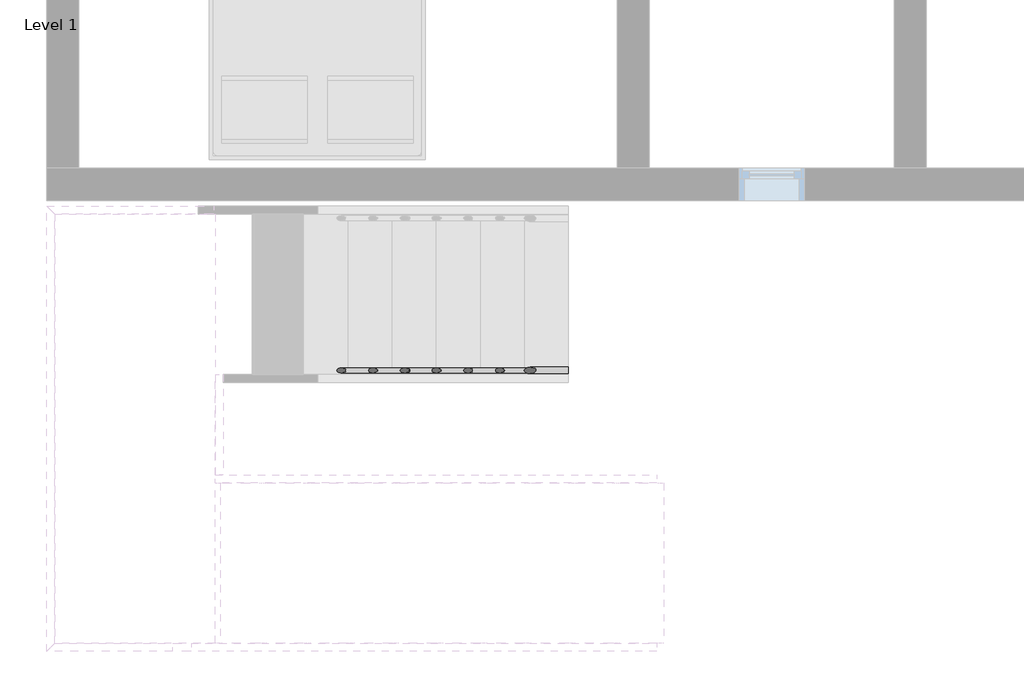
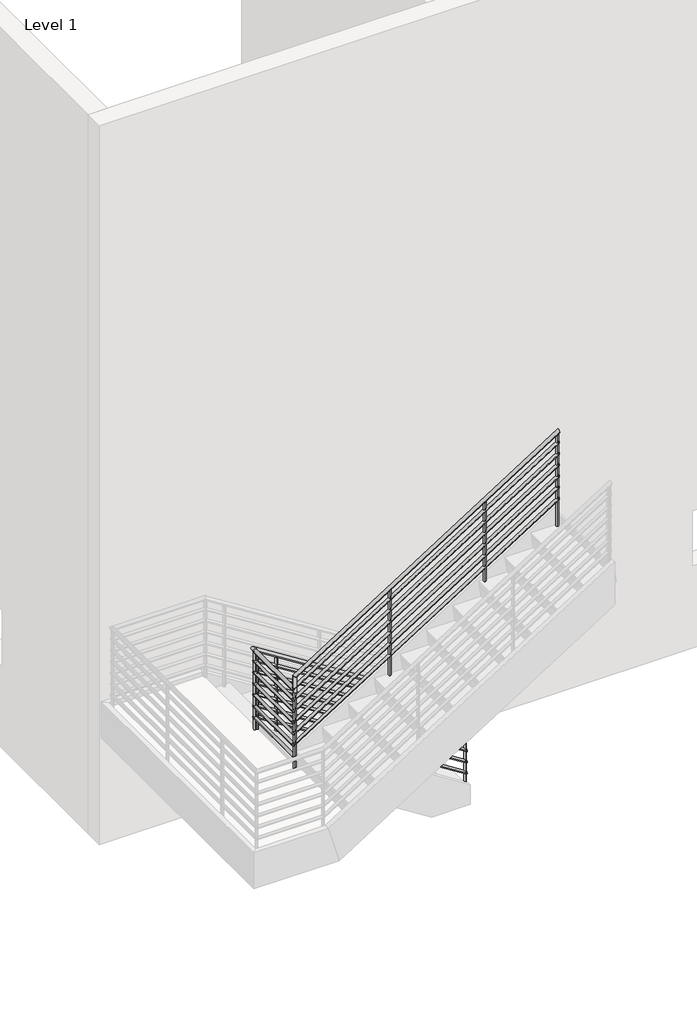
# One storey, part 3 of 4: 1 railing.
"""IFC4 building model written with IfcOpenShell, lengths in millimetres."""

from ifc_helpers import new_model, si_unit, point, frame, frame_2d, origin, place, context, project, spatial, circle_curve, ellipse_curve, trimmed, segment, composite_curve, outline, extrude, element, save
from ifc_brep_helpers import plane_surface, cylinder_surface, advanced_brep

model = new_model("IFC4")

# Units and contexts
model_context = context("Model", 3, world=origin())
ifc_project = project(units=[si_unit("LENGTHUNIT", "METRE", prefix="MILLI")], contexts=[model_context])

# Site, building, storey
site = spatial("IfcSite", under=ifc_project)
building = spatial("IfcBuilding", under=site)
storey = spatial("IfcBuildingStorey", under=building, Name="Level 1", Elevation=0.0)

# Railing
placement = place(None, origin())
element("IfcRailing", 1, ObjectType="900mm Pipe", at=placement, inside=storey, context=model_context, shape_type="SolidModel", body=[
    advanced_brep(
    [(-8274.8492596, 5292.330447, 1050.2491997), (-8274.8492596, 5252.330447, 1050.2491997), (-10527.842597, 5292.330447, 2475.0671206), (-10494.0357478, 5252.330447, 2453.687295)],
    [
        (0, 1, ellipse_curve(frame((-8274.8492596, 5272.330447, 1050.2491997), z_axis=(1.0, 0.0, 0.0), x_axis=(0.0, 0.0, -1.0)), 23.6638438, 20.0)),
        (1, 0, ellipse_curve(frame((-8274.8492596, 5272.330447, 1050.2491997), z_axis=(1.0, 0.0, 0.0), x_axis=(0.0, 0.0, -1.0)), 23.6638438, 20.0)),
        (2, 3, ellipse_curve(frame((-10510.9391724, 5272.330447, 2464.3772078), z_axis=(-0.5976263089853407, -0.7071067811865477, 0.3779454918484382), x_axis=(0.5976263089853421, -0.7071067811865474, -0.3779454918484364)), 28.2842712, 20.0)),
        (3, 2, ellipse_curve(frame((-10510.9391724, 5272.330447, 2464.3772078), z_axis=(-0.5976263089853407, -0.7071067811865477, 0.3779454918484382), x_axis=(0.5976263089853421, -0.7071067811865474, -0.3779454918484364)), 28.2842712, 20.0)),
        (0, 2),
        (3, 1),
    ],
    [
        plane_surface(frame((-8274.8492596, 5272.330447, 1073.9130435), z_axis=(1.0, 0.0, 0.0), x_axis=(0.0, -1.0, 0.0))),
        plane_surface(frame((-10500.2492596, 5272.330447, 2481.2806324), z_axis=(-0.5976263089853409, -0.7071067811865478, 0.3779454918484383), x_axis=(0.8017747781070181, -0.5270627453469436, 0.28171273961037846))),
        cylinder_surface(frame((-8285.5391724, 5272.330447, 1057.0096189), z_axis=(0.8451712313980438, 0.0, -0.5344956404098301), x_axis=(0.0, -1.0, 0.0)), 20.0),
    ],
    [
        (0, [[1, 2]]),
        (1, [[3, 4]]),
        (2, [[-1, 5, -4, 6]]),
        (2, [[-2, -6, -3, -5]]),
    ],
),
    advanced_brep(
    [(-10520.2492596, 5278.5439589, 2445.2173913), (-10480.2492596, 5244.7371096, 2445.2173913), (-10520.2492596, 4545.1562283, 2445.2173913), (-10480.2492596, 4545.1562283, 2445.2173913)],
    [
        (0, 1, ellipse_curve(frame((-10500.2492596, 5261.6405342, 2445.2173913), z_axis=(0.5976263089853407, 0.7071067811865477, -0.3779454918484382), x_axis=(-0.5976263089853423, 0.7071067811865472, 0.3779454918484363)), 28.2842712, 20.0)),
        (1, 0, ellipse_curve(frame((-10500.2492596, 5261.6405342, 2445.2173913), z_axis=(0.5976263089853407, 0.7071067811865477, -0.3779454918484382), x_axis=(-0.5976263089853423, 0.7071067811865472, 0.3779454918484363)), 28.2842712, 20.0)),
        (2, 3, ellipse_curve(frame((-10500.2492596, 4545.1562283, 2445.2173913), z_axis=(0.0, -0.7071067811865476, 0.7071067811865476), x_axis=(0.0, 0.7071067811865474, 0.7071067811865476)), 28.2842712, 20.0)),
        (3, 2, ellipse_curve(frame((-10500.2492596, 4545.1562283, 2445.2173913), z_axis=(0.0, -0.7071067811865476, 0.7071067811865476), x_axis=(0.0, 0.7071067811865474, 0.7071067811865476)), 28.2842712, 20.0)),
        (0, 2),
        (3, 1),
    ],
    [
        plane_surface(frame((-10500.2492596, 5272.330447, 2465.2173913), z_axis=(0.5976263089853409, 0.7071067811865478, -0.3779454918484383), x_axis=(0.8017747781070181, -0.5270627453469436, 0.28171273961037846))),
        plane_surface(frame((-10500.2492596, 4565.1562283, 2465.2173913), z_axis=(0.0, -0.7071067811865476, 0.7071067811865476), x_axis=(1.0, 0.0, 0.0))),
        cylinder_surface(frame((-10500.2492596, 5272.330447, 2445.2173913), z_axis=(0.0, 1.0, 0.0), x_axis=(1.0, 0.0, 0.0)), 20.0),
    ],
    [
        (0, [[1, 2]]),
        (1, [[3, 4]]),
        (2, [[-1, 5, -4, 6]]),
        (2, [[-2, -6, -3, -5]]),
    ],
),
    advanced_brep(
    [(-10500.2492596, 4525.1562283, 2599.4033499), (-10500.2492596, 4565.1562283, 2599.4033499), (-7724.8492596, 4525.1562283, 4354.5970258), (-7724.8492596, 4565.1562283, 4354.5970258)],
    [
        (0, 1, ellipse_curve(frame((-10500.2492596, 4545.1562283, 2599.4033499), z_axis=(-0.4824439654458175, 0.0, -0.8759268349610685), x_axis=(-0.8759268349610684, 0.0, 0.48244396544581764)), 22.8329573, 20.0)),
        (1, 0, ellipse_curve(frame((-10500.2492596, 4545.1562283, 2599.4033499), z_axis=(-0.4824439654458175, 0.0, -0.8759268349610685), x_axis=(-0.8759268349610684, 0.0, 0.48244396544581764)), 22.8329573, 20.0)),
        (2, 3, ellipse_curve(frame((-7724.8492596, 4545.1562283, 4354.5970258), z_axis=(1.0, 0.0, 0.0), x_axis=(0.0, 0.0, -1.0)), 23.6638438, 20.0)),
        (3, 2, ellipse_curve(frame((-7724.8492596, 4545.1562283, 4354.5970258), z_axis=(1.0, 0.0, 0.0), x_axis=(0.0, 0.0, -1.0)), 23.6638438, 20.0)),
        (0, 2),
        (3, 1),
    ],
    [
        plane_surface(frame((-10520.2492596, 4545.1562283, 2610.4189723), z_axis=(-0.4824439654458175, 0.0, -0.8759268349610685), x_axis=(0.8759268349610685, 0.0, -0.4824439654458175))),
        plane_surface(frame((-7724.8492596, 4545.1562283, 4378.2608696), z_axis=(1.0, 0.0, 0.0), x_axis=(0.0, 1.0, 0.0))),
        cylinder_surface(frame((-10509.5593468, 4545.1562283, 2593.5155477), z_axis=(-0.8451712313980441, 0.0, -0.5344956404098298), x_axis=(0.0, 1.0, 0.0)), 20.0),
    ],
    [
        (0, [[1, 2]]),
        (1, [[3, 4]]),
        (2, [[-1, 5, -4, 6]]),
        (2, [[-2, -6, -3, -5]]),
    ],
),
    advanced_brep(
    [(-10520.2492596, 4545.1562283, 2445.2173913), (-10480.2492596, 4545.1562283, 2445.2173913), (-10520.2492596, 4545.1562283, 2610.4189723), (-10480.2492596, 4545.1562283, 2588.3877274)],
    [
        (0, 1, ellipse_curve(frame((-10500.2492596, 4545.1562283, 2445.2173913), z_axis=(0.0, 0.7071067811865476, -0.7071067811865476), x_axis=(0.0, -0.7071067811865476, -0.7071067811865474)), 28.2842712, 20.0)),
        (1, 0, ellipse_curve(frame((-10500.2492596, 4545.1562283, 2445.2173913), z_axis=(0.0, 0.7071067811865476, -0.7071067811865476), x_axis=(0.0, -0.7071067811865476, -0.7071067811865474)), 28.2842712, 20.0)),
        (2, 3, ellipse_curve(frame((-10500.2492596, 4545.1562283, 2599.4033499), z_axis=(0.4824439654458175, 0.0, 0.8759268349610685), x_axis=(0.8759268349610685, 0.0, -0.4824439654458174)), 22.8329573, 20.0)),
        (3, 2, ellipse_curve(frame((-10500.2492596, 4545.1562283, 2599.4033499), z_axis=(0.4824439654458175, 0.0, 0.8759268349610685), x_axis=(0.8759268349610685, 0.0, -0.4824439654458174)), 22.8329573, 20.0)),
        (0, 2),
        (3, 1),
    ],
    [
        plane_surface(frame((-10500.2492596, 4545.1562283, 2445.2173913), z_axis=(0.0, 0.7071067811865476, -0.7071067811865476), x_axis=(1.0, 0.0, 0.0))),
        plane_surface(frame((-10500.2492596, 4545.1562283, 2599.4033499), z_axis=(0.4824439654458175, 0.0, 0.8759268349610685), x_axis=(0.8759268349610685, 0.0, -0.4824439654458175))),
        cylinder_surface(frame((-10500.2492596, 4545.1562283, 2445.2173913), z_axis=(0.0, 0.0, -1.0), x_axis=(1.0, 0.0, 0.0)), 20.0),
    ],
    [
        (0, [[1, 2]]),
        (1, [[3, 4]]),
        (2, [[-1, 5, -4, 6]]),
        (2, [[-2, -6, -3, -5]]),
    ],
),
    advanced_brep(
    [(-8274.8492596, 5287.330447, 931.1651606), (-8274.8492596, 5257.330447, 931.1651606), (-10479.1943493, 5287.330447, 2325.2173913), (-10479.1943493, 5257.330447, 2325.2173913), (-10515.2492596, 5287.330447, 2325.2173913), (-10485.2492596, 5257.330447, 2325.2173913), (-10515.2492596, 4560.1562283, 2325.2173913), (-10485.2492596, 4560.1562283, 2325.2173913)],
    [
        (0, 1, ellipse_curve(frame((-8274.8492596, 5272.330447, 931.1651606), z_axis=(1.0, 0.0, 0.0), x_axis=(0.0, 0.0, -1.0)), 17.7478828, 15.0)),
        (1, 0, ellipse_curve(frame((-8274.8492596, 5272.330447, 931.1651606), z_axis=(1.0, 0.0, 0.0), x_axis=(0.0, 0.0, -1.0)), 17.7478828, 15.0)),
        (0, 2),
        (2, 3, ellipse_curve(frame((-10479.1943493, 5272.330447, 2325.2173913), z_axis=(0.9605132043335072, 0.0, -0.2782344053149755), x_axis=(-0.2782344053149752, 0.0, -0.9605132043335075)), 15.6166515, 15.0)),
        (3, 1),
        (3, 2, ellipse_curve(frame((-10479.1943493, 5272.330447, 2325.2173913), z_axis=(0.9605132043335072, 0.0, -0.2782344053149755), x_axis=(-0.2782344053149752, 0.0, -0.9605132043335075)), 15.6166515, 15.0)),
        (2, 4),
        (4, 5, ellipse_curve(frame((-10500.2492596, 5272.330447, 2325.2173913), z_axis=(0.7071067811865474, 0.7071067811865476, 0.0), x_axis=(0.7071067811865478, -0.7071067811865472, 0.0)), 21.2132034, 15.0)),
        (5, 3),
        (5, 4, ellipse_curve(frame((-10500.2492596, 5272.330447, 2325.2173913), z_axis=(0.7071067811865474, 0.7071067811865476, 0.0), x_axis=(0.7071067811865478, -0.7071067811865472, 0.0)), 21.2132034, 15.0)),
        (6, 7, circle_curve(frame((-10500.2492596, 4560.1562283, 2325.2173913), z_axis=(0.0, -1.0, 0.0), x_axis=(1.0, 0.0, 0.0)), 15.0)),
        (7, 6, circle_curve(frame((-10500.2492596, 4560.1562283, 2325.2173913), z_axis=(0.0, -1.0, 0.0), x_axis=(1.0, 0.0, 0.0)), 15.0)),
        (4, 6),
        (7, 5),
    ],
    [
        plane_surface(frame((-8274.8492596, 5272.330447, 948.9130435), z_axis=(1.0, 0.0, 0.0), x_axis=(0.0, -1.0, 0.0))),
        cylinder_surface(frame((-8282.8666942, 5272.330447, 936.235475), z_axis=(0.8451712313980437, 0.0, -0.5344956404098301), x_axis=(0.0, -1.0, 0.0)), 15.0),
        cylinder_surface(frame((-10474.8492596, 5272.330447, 2325.2173913), z_axis=(1.0, 0.0, 0.0), x_axis=(0.0, -1.0, 0.0)), 15.0),
        plane_surface(frame((-10500.2492596, 4560.1562283, 2340.2173913), z_axis=(0.0, -1.0, 0.0), x_axis=(0.0, 0.0, -1.0))),
        cylinder_surface(frame((-10500.2492596, 5272.330447, 2325.2173913), z_axis=(0.0, 1.0, 0.0), x_axis=(1.0, 0.0, 0.0)), 15.0),
    ],
    [
        (0, [[1, 2]]),
        (1, [[-1, 3, 4, 5]]),
        (1, [[-2, -5, 6, -3]]),
        (2, [[-4, 7, 8, 9]]),
        (2, [[-6, -9, 10, -7]]),
        (3, [[11, 12]]),
        (4, [[-8, 13, -12, 14]]),
        (4, [[-10, -14, -11, -13]]),
    ],
),
    advanced_brep(
    [(-10515.2492596, 4530.1562283, 2470.8331448), (-10515.2492596, 4560.1562283, 2470.8331448), (-7724.8492596, 4530.1562283, 4235.5129867), (-7724.8492596, 4560.1562283, 4235.5129867)],
    [
        (0, 1, ellipse_curve(frame((-10515.2492596, 4545.1562283, 2470.8331448), z_axis=(-1.0, 0.0, 0.0), x_axis=(0.0, 0.0, -1.0)), 17.7478828, 15.0)),
        (1, 0, ellipse_curve(frame((-10515.2492596, 4545.1562283, 2470.8331448), z_axis=(-1.0, 0.0, 0.0), x_axis=(0.0, 0.0, -1.0)), 17.7478828, 15.0)),
        (2, 3, ellipse_curve(frame((-7724.8492596, 4545.1562283, 4235.5129867), z_axis=(1.0, 0.0, 0.0), x_axis=(0.0, 0.0, -1.0)), 17.7478828, 15.0)),
        (3, 2, ellipse_curve(frame((-7724.8492596, 4545.1562283, 4235.5129867), z_axis=(1.0, 0.0, 0.0), x_axis=(0.0, 0.0, -1.0)), 17.7478828, 15.0)),
        (0, 2),
        (3, 1),
    ],
    [
        plane_surface(frame((-10515.2492596, 4545.1562283, 2488.5810277), z_axis=(-1.0, 0.0, 0.0), x_axis=(0.0, 1.0, 0.0))),
        plane_surface(frame((-7724.8492596, 4545.1562283, 4253.2608696), z_axis=(1.0, 0.0, 0.0), x_axis=(0.0, 1.0, 0.0))),
        cylinder_surface(frame((-10507.231825, 4545.1562283, 2475.9034592), z_axis=(-0.8451712313980441, 0.0, -0.5344956404098298), x_axis=(0.0, 1.0, 0.0)), 15.0),
    ],
    [
        (0, [[1, 2]]),
        (1, [[3, 4]]),
        (2, [[-1, 5, -4, 6]]),
        (2, [[-2, -6, -3, -5]]),
    ],
),
    advanced_brep(
    [(-8274.8492596, 5287.330447, 806.1651606), (-8274.8492596, 5257.330447, 806.1651606), (-10479.1943493, 5287.330447, 2200.2173913), (-10479.1943493, 5257.330447, 2200.2173913), (-10515.2492596, 5287.330447, 2200.2173913), (-10485.2492596, 5257.330447, 2200.2173913), (-10515.2492596, 4560.1562283, 2200.2173913), (-10485.2492596, 4560.1562283, 2200.2173913)],
    [
        (0, 1, ellipse_curve(frame((-8274.8492596, 5272.330447, 806.1651606), z_axis=(1.0, 0.0, 0.0), x_axis=(0.0, 0.0, -1.0)), 17.7478828, 15.0)),
        (1, 0, ellipse_curve(frame((-8274.8492596, 5272.330447, 806.1651606), z_axis=(1.0, 0.0, 0.0), x_axis=(0.0, 0.0, -1.0)), 17.7478828, 15.0)),
        (0, 2),
        (2, 3, ellipse_curve(frame((-10479.1943493, 5272.330447, 2200.2173913), z_axis=(0.9605132043335072, 0.0, -0.2782344053149755), x_axis=(-0.2782344053149752, 0.0, -0.9605132043335075)), 15.6166515, 15.0)),
        (3, 1),
        (3, 2, ellipse_curve(frame((-10479.1943493, 5272.330447, 2200.2173913), z_axis=(0.9605132043335072, 0.0, -0.2782344053149755), x_axis=(-0.2782344053149752, 0.0, -0.9605132043335075)), 15.6166515, 15.0)),
        (2, 4),
        (4, 5, ellipse_curve(frame((-10500.2492596, 5272.330447, 2200.2173913), z_axis=(0.7071067811865474, 0.7071067811865476, 0.0), x_axis=(0.7071067811865478, -0.7071067811865472, 0.0)), 21.2132034, 15.0)),
        (5, 3),
        (5, 4, ellipse_curve(frame((-10500.2492596, 5272.330447, 2200.2173913), z_axis=(0.7071067811865474, 0.7071067811865476, 0.0), x_axis=(0.7071067811865478, -0.7071067811865472, 0.0)), 21.2132034, 15.0)),
        (6, 7, circle_curve(frame((-10500.2492596, 4560.1562283, 2200.2173913), z_axis=(0.0, -1.0, 0.0), x_axis=(1.0, 0.0, 0.0)), 15.0)),
        (7, 6, circle_curve(frame((-10500.2492596, 4560.1562283, 2200.2173913), z_axis=(0.0, -1.0, 0.0), x_axis=(1.0, 0.0, 0.0)), 15.0)),
        (4, 6),
        (7, 5),
    ],
    [
        plane_surface(frame((-8274.8492596, 5272.330447, 823.9130435), z_axis=(1.0, 0.0, 0.0), x_axis=(0.0, -1.0, 0.0))),
        cylinder_surface(frame((-8282.8666942, 5272.330447, 811.235475), z_axis=(0.8451712313980437, 0.0, -0.5344956404098301), x_axis=(0.0, -1.0, 0.0)), 15.0),
        cylinder_surface(frame((-10474.8492596, 5272.330447, 2200.2173913), z_axis=(1.0, 0.0, 0.0), x_axis=(0.0, -1.0, 0.0)), 15.0),
        plane_surface(frame((-10500.2492596, 4560.1562283, 2215.2173913), z_axis=(0.0, -1.0, 0.0), x_axis=(0.0, 0.0, -1.0))),
        cylinder_surface(frame((-10500.2492596, 5272.330447, 2200.2173913), z_axis=(0.0, 1.0, 0.0), x_axis=(1.0, 0.0, 0.0)), 15.0),
    ],
    [
        (0, [[1, 2]]),
        (1, [[-1, 3, 4, 5]]),
        (1, [[-2, -5, 6, -3]]),
        (2, [[-4, 7, 8, 9]]),
        (2, [[-6, -9, 10, -7]]),
        (3, [[11, 12]]),
        (4, [[-8, 13, -12, 14]]),
        (4, [[-10, -14, -11, -13]]),
    ],
),
    advanced_brep(
    [(-10515.2492596, 4530.1562283, 2345.8331448), (-10515.2492596, 4560.1562283, 2345.8331448), (-7724.8492596, 4530.1562283, 4110.5129867), (-7724.8492596, 4560.1562283, 4110.5129867)],
    [
        (0, 1, ellipse_curve(frame((-10515.2492596, 4545.1562283, 2345.8331448), z_axis=(-1.0, 0.0, 0.0), x_axis=(0.0, 0.0, -1.0)), 17.7478828, 15.0)),
        (1, 0, ellipse_curve(frame((-10515.2492596, 4545.1562283, 2345.8331448), z_axis=(-1.0, 0.0, 0.0), x_axis=(0.0, 0.0, -1.0)), 17.7478828, 15.0)),
        (2, 3, ellipse_curve(frame((-7724.8492596, 4545.1562283, 4110.5129867), z_axis=(1.0, 0.0, 0.0), x_axis=(0.0, 0.0, -1.0)), 17.7478828, 15.0)),
        (3, 2, ellipse_curve(frame((-7724.8492596, 4545.1562283, 4110.5129867), z_axis=(1.0, 0.0, 0.0), x_axis=(0.0, 0.0, -1.0)), 17.7478828, 15.0)),
        (0, 2),
        (3, 1),
    ],
    [
        plane_surface(frame((-10515.2492596, 4545.1562283, 2363.5810277), z_axis=(-1.0, 0.0, 0.0), x_axis=(0.0, 1.0, 0.0))),
        plane_surface(frame((-7724.8492596, 4545.1562283, 4128.2608696), z_axis=(1.0, 0.0, 0.0), x_axis=(0.0, 1.0, 0.0))),
        cylinder_surface(frame((-10507.231825, 4545.1562283, 2350.9034592), z_axis=(-0.8451712313980441, 0.0, -0.5344956404098297), x_axis=(0.0, 1.0, 0.0)), 15.0),
    ],
    [
        (0, [[1, 2]]),
        (1, [[3, 4]]),
        (2, [[-1, 5, -4, 6]]),
        (2, [[-2, -6, -3, -5]]),
    ],
),
    advanced_brep(
    [(-8274.8492596, 5287.330447, 681.1651606), (-8274.8492596, 5257.330447, 681.1651606), (-10479.1943493, 5287.330447, 2075.2173913), (-10479.1943493, 5257.330447, 2075.2173913), (-10515.2492596, 5287.330447, 2075.2173913), (-10485.2492596, 5257.330447, 2075.2173913), (-10515.2492596, 4560.1562283, 2075.2173913), (-10485.2492596, 4560.1562283, 2075.2173913)],
    [
        (0, 1, ellipse_curve(frame((-8274.8492596, 5272.330447, 681.1651606), z_axis=(1.0, 0.0, 0.0), x_axis=(0.0, 0.0, -1.0)), 17.7478828, 15.0)),
        (1, 0, ellipse_curve(frame((-8274.8492596, 5272.330447, 681.1651606), z_axis=(1.0, 0.0, 0.0), x_axis=(0.0, 0.0, -1.0)), 17.7478828, 15.0)),
        (0, 2),
        (2, 3, ellipse_curve(frame((-10479.1943493, 5272.330447, 2075.2173913), z_axis=(0.9605132043335072, 0.0, -0.2782344053149755), x_axis=(-0.2782344053149752, 0.0, -0.9605132043335075)), 15.6166515, 15.0)),
        (3, 1),
        (3, 2, ellipse_curve(frame((-10479.1943493, 5272.330447, 2075.2173913), z_axis=(0.9605132043335072, 0.0, -0.2782344053149755), x_axis=(-0.2782344053149752, 0.0, -0.9605132043335075)), 15.6166515, 15.0)),
        (2, 4),
        (4, 5, ellipse_curve(frame((-10500.2492596, 5272.330447, 2075.2173913), z_axis=(0.7071067811865474, 0.7071067811865476, 0.0), x_axis=(0.7071067811865478, -0.7071067811865472, 0.0)), 21.2132034, 15.0)),
        (5, 3),
        (5, 4, ellipse_curve(frame((-10500.2492596, 5272.330447, 2075.2173913), z_axis=(0.7071067811865474, 0.7071067811865476, 0.0), x_axis=(0.7071067811865478, -0.7071067811865472, 0.0)), 21.2132034, 15.0)),
        (6, 7, circle_curve(frame((-10500.2492596, 4560.1562283, 2075.2173913), z_axis=(0.0, -1.0, 0.0), x_axis=(1.0, 0.0, 0.0)), 15.0)),
        (7, 6, circle_curve(frame((-10500.2492596, 4560.1562283, 2075.2173913), z_axis=(0.0, -1.0, 0.0), x_axis=(1.0, 0.0, 0.0)), 15.0)),
        (4, 6),
        (7, 5),
    ],
    [
        plane_surface(frame((-8274.8492596, 5272.330447, 698.9130435), z_axis=(1.0, 0.0, 0.0), x_axis=(0.0, -1.0, 0.0))),
        cylinder_surface(frame((-8282.8666942, 5272.330447, 686.235475), z_axis=(0.8451712313980437, 0.0, -0.5344956404098301), x_axis=(0.0, -1.0, 0.0)), 15.0),
        cylinder_surface(frame((-10474.8492596, 5272.330447, 2075.2173913), z_axis=(1.0, 0.0, 0.0), x_axis=(0.0, -1.0, 0.0)), 15.0),
        plane_surface(frame((-10500.2492596, 4560.1562283, 2090.2173913), z_axis=(0.0, -1.0, 0.0), x_axis=(0.0, 0.0, -1.0))),
        cylinder_surface(frame((-10500.2492596, 5272.330447, 2075.2173913), z_axis=(0.0, 1.0, 0.0), x_axis=(1.0, 0.0, 0.0)), 15.0),
    ],
    [
        (0, [[1, 2]]),
        (1, [[-1, 3, 4, 5]]),
        (1, [[-2, -5, 6, -3]]),
        (2, [[-4, 7, 8, 9]]),
        (2, [[-6, -9, 10, -7]]),
        (3, [[11, 12]]),
        (4, [[-8, 13, -12, 14]]),
        (4, [[-10, -14, -11, -13]]),
    ],
),
    advanced_brep(
    [(-10515.2492596, 4530.1562283, 2220.8331448), (-10515.2492596, 4560.1562283, 2220.8331448), (-7724.8492596, 4530.1562283, 3985.5129867), (-7724.8492596, 4560.1562283, 3985.5129867)],
    [
        (0, 1, ellipse_curve(frame((-10515.2492596, 4545.1562283, 2220.8331448), z_axis=(-1.0, 0.0, 0.0), x_axis=(0.0, 0.0, -1.0)), 17.7478828, 15.0)),
        (1, 0, ellipse_curve(frame((-10515.2492596, 4545.1562283, 2220.8331448), z_axis=(-1.0, 0.0, 0.0), x_axis=(0.0, 0.0, -1.0)), 17.7478828, 15.0)),
        (2, 3, ellipse_curve(frame((-7724.8492596, 4545.1562283, 3985.5129867), z_axis=(1.0, 0.0, 0.0), x_axis=(0.0, 0.0, -1.0)), 17.7478828, 15.0)),
        (3, 2, ellipse_curve(frame((-7724.8492596, 4545.1562283, 3985.5129867), z_axis=(1.0, 0.0, 0.0), x_axis=(0.0, 0.0, -1.0)), 17.7478828, 15.0)),
        (0, 2),
        (3, 1),
    ],
    [
        plane_surface(frame((-10515.2492596, 4545.1562283, 2238.5810277), z_axis=(-1.0, 0.0, 0.0), x_axis=(0.0, 1.0, 0.0))),
        plane_surface(frame((-7724.8492596, 4545.1562283, 4003.2608696), z_axis=(1.0, 0.0, 0.0), x_axis=(0.0, 1.0, 0.0))),
        cylinder_surface(frame((-10507.231825, 4545.1562283, 2225.9034592), z_axis=(-0.8451712313980441, 0.0, -0.5344956404098296), x_axis=(0.0, 1.0, 0.0)), 15.0),
    ],
    [
        (0, [[1, 2]]),
        (1, [[3, 4]]),
        (2, [[-1, 5, -4, 6]]),
        (2, [[-2, -6, -3, -5]]),
    ],
),
    advanced_brep(
    [(-8274.8492596, 5287.330447, 556.1651606), (-8274.8492596, 5257.330447, 556.1651606), (-10479.1943493, 5287.330447, 1950.2173913), (-10479.1943493, 5257.330447, 1950.2173913), (-10515.2492596, 5287.330447, 1950.2173913), (-10485.2492596, 5257.330447, 1950.2173913), (-10515.2492596, 4560.1562283, 1950.2173913), (-10485.2492596, 4560.1562283, 1950.2173913)],
    [
        (0, 1, ellipse_curve(frame((-8274.8492596, 5272.330447, 556.1651606), z_axis=(1.0, 0.0, 0.0), x_axis=(0.0, 0.0, -1.0)), 17.7478828, 15.0)),
        (1, 0, ellipse_curve(frame((-8274.8492596, 5272.330447, 556.1651606), z_axis=(1.0, 0.0, 0.0), x_axis=(0.0, 0.0, -1.0)), 17.7478828, 15.0)),
        (0, 2),
        (2, 3, ellipse_curve(frame((-10479.1943493, 5272.330447, 1950.2173913), z_axis=(0.9605132043335072, 0.0, -0.2782344053149755), x_axis=(-0.2782344053149752, 0.0, -0.9605132043335075)), 15.6166515, 15.0)),
        (3, 1),
        (3, 2, ellipse_curve(frame((-10479.1943493, 5272.330447, 1950.2173913), z_axis=(0.9605132043335072, 0.0, -0.2782344053149755), x_axis=(-0.2782344053149752, 0.0, -0.9605132043335075)), 15.6166515, 15.0)),
        (2, 4),
        (4, 5, ellipse_curve(frame((-10500.2492596, 5272.330447, 1950.2173913), z_axis=(0.7071067811865474, 0.7071067811865476, 0.0), x_axis=(0.7071067811865478, -0.7071067811865472, 0.0)), 21.2132034, 15.0)),
        (5, 3),
        (5, 4, ellipse_curve(frame((-10500.2492596, 5272.330447, 1950.2173913), z_axis=(0.7071067811865474, 0.7071067811865476, 0.0), x_axis=(0.7071067811865478, -0.7071067811865472, 0.0)), 21.2132034, 15.0)),
        (6, 7, circle_curve(frame((-10500.2492596, 4560.1562283, 1950.2173913), z_axis=(0.0, -1.0, 0.0), x_axis=(1.0, 0.0, 0.0)), 15.0)),
        (7, 6, circle_curve(frame((-10500.2492596, 4560.1562283, 1950.2173913), z_axis=(0.0, -1.0, 0.0), x_axis=(1.0, 0.0, 0.0)), 15.0)),
        (4, 6),
        (7, 5),
    ],
    [
        plane_surface(frame((-8274.8492596, 5272.330447, 573.9130435), z_axis=(1.0, 0.0, 0.0), x_axis=(0.0, -1.0, 0.0))),
        cylinder_surface(frame((-8282.8666942, 5272.330447, 561.235475), z_axis=(0.8451712313980437, 0.0, -0.5344956404098301), x_axis=(0.0, -1.0, 0.0)), 15.0),
        cylinder_surface(frame((-10474.8492596, 5272.330447, 1950.2173913), z_axis=(1.0, 0.0, 0.0), x_axis=(0.0, -1.0, 0.0)), 15.0),
        plane_surface(frame((-10500.2492596, 4560.1562283, 1965.2173913), z_axis=(0.0, -1.0, 0.0), x_axis=(0.0, 0.0, -1.0))),
        cylinder_surface(frame((-10500.2492596, 5272.330447, 1950.2173913), z_axis=(0.0, 1.0, 0.0), x_axis=(1.0, 0.0, 0.0)), 15.0),
    ],
    [
        (0, [[1, 2]]),
        (1, [[-1, 3, 4, 5]]),
        (1, [[-2, -5, 6, -3]]),
        (2, [[-4, 7, 8, 9]]),
        (2, [[-6, -9, 10, -7]]),
        (3, [[11, 12]]),
        (4, [[-8, 13, -12, 14]]),
        (4, [[-10, -14, -11, -13]]),
    ],
),
    advanced_brep(
    [(-10515.2492596, 4530.1562283, 2095.8331448), (-10515.2492596, 4560.1562283, 2095.8331448), (-7724.8492596, 4530.1562283, 3860.5129867), (-7724.8492596, 4560.1562283, 3860.5129867)],
    [
        (0, 1, ellipse_curve(frame((-10515.2492596, 4545.1562283, 2095.8331448), z_axis=(-1.0, 0.0, 0.0), x_axis=(0.0, 0.0, -1.0)), 17.7478828, 15.0)),
        (1, 0, ellipse_curve(frame((-10515.2492596, 4545.1562283, 2095.8331448), z_axis=(-1.0, 0.0, 0.0), x_axis=(0.0, 0.0, -1.0)), 17.7478828, 15.0)),
        (2, 3, ellipse_curve(frame((-7724.8492596, 4545.1562283, 3860.5129867), z_axis=(1.0, 0.0, 0.0), x_axis=(0.0, 0.0, -1.0)), 17.7478828, 15.0)),
        (3, 2, ellipse_curve(frame((-7724.8492596, 4545.1562283, 3860.5129867), z_axis=(1.0, 0.0, 0.0), x_axis=(0.0, 0.0, -1.0)), 17.7478828, 15.0)),
        (0, 2),
        (3, 1),
    ],
    [
        plane_surface(frame((-10515.2492596, 4545.1562283, 2113.5810277), z_axis=(-1.0, 0.0, 0.0), x_axis=(0.0, 1.0, 0.0))),
        plane_surface(frame((-7724.8492596, 4545.1562283, 3878.2608696), z_axis=(1.0, 0.0, 0.0), x_axis=(0.0, 1.0, 0.0))),
        cylinder_surface(frame((-10507.231825, 4545.1562283, 2100.9034592), z_axis=(-0.8451712313980441, 0.0, -0.5344956404098297), x_axis=(0.0, 1.0, 0.0)), 15.0),
    ],
    [
        (0, [[1, 2]]),
        (1, [[3, 4]]),
        (2, [[-1, 5, -4, 6]]),
        (2, [[-2, -6, -3, -5]]),
    ],
),
    advanced_brep(
    [(-8274.8492596, 5287.330447, 431.1651606), (-8274.8492596, 5257.330447, 431.1651606), (-10479.1943493, 5287.330447, 1825.2173913), (-10479.1943493, 5257.330447, 1825.2173913), (-10515.2492596, 5287.330447, 1825.2173913), (-10485.2492596, 5257.330447, 1825.2173913), (-10515.2492596, 4560.1562283, 1825.2173913), (-10485.2492596, 4560.1562283, 1825.2173913)],
    [
        (0, 1, ellipse_curve(frame((-8274.8492596, 5272.330447, 431.1651606), z_axis=(1.0, 0.0, 0.0), x_axis=(0.0, 0.0, -1.0)), 17.7478828, 15.0)),
        (1, 0, ellipse_curve(frame((-8274.8492596, 5272.330447, 431.1651606), z_axis=(1.0, 0.0, 0.0), x_axis=(0.0, 0.0, -1.0)), 17.7478828, 15.0)),
        (0, 2),
        (2, 3, ellipse_curve(frame((-10479.1943493, 5272.330447, 1825.2173913), z_axis=(0.9605132043335072, 0.0, -0.2782344053149755), x_axis=(-0.2782344053149752, 0.0, -0.9605132043335075)), 15.6166515, 15.0)),
        (3, 1),
        (3, 2, ellipse_curve(frame((-10479.1943493, 5272.330447, 1825.2173913), z_axis=(0.9605132043335072, 0.0, -0.2782344053149755), x_axis=(-0.2782344053149752, 0.0, -0.9605132043335075)), 15.6166515, 15.0)),
        (2, 4),
        (4, 5, ellipse_curve(frame((-10500.2492596, 5272.330447, 1825.2173913), z_axis=(0.7071067811865474, 0.7071067811865476, 0.0), x_axis=(0.7071067811865478, -0.7071067811865472, 0.0)), 21.2132034, 15.0)),
        (5, 3),
        (5, 4, ellipse_curve(frame((-10500.2492596, 5272.330447, 1825.2173913), z_axis=(0.7071067811865474, 0.7071067811865476, 0.0), x_axis=(0.7071067811865478, -0.7071067811865472, 0.0)), 21.2132034, 15.0)),
        (6, 7, circle_curve(frame((-10500.2492596, 4560.1562283, 1825.2173913), z_axis=(0.0, -1.0, 0.0), x_axis=(1.0, 0.0, 0.0)), 15.0)),
        (7, 6, circle_curve(frame((-10500.2492596, 4560.1562283, 1825.2173913), z_axis=(0.0, -1.0, 0.0), x_axis=(1.0, 0.0, 0.0)), 15.0)),
        (4, 6),
        (7, 5),
    ],
    [
        plane_surface(frame((-8274.8492596, 5272.330447, 448.9130435), z_axis=(1.0, 0.0, 0.0), x_axis=(0.0, -1.0, 0.0))),
        cylinder_surface(frame((-8282.8666942, 5272.330447, 436.235475), z_axis=(0.8451712313980437, 0.0, -0.5344956404098301), x_axis=(0.0, -1.0, 0.0)), 15.0),
        cylinder_surface(frame((-10474.8492596, 5272.330447, 1825.2173913), z_axis=(1.0, 0.0, 0.0), x_axis=(0.0, -1.0, 0.0)), 15.0),
        plane_surface(frame((-10500.2492596, 4560.1562283, 1840.2173913), z_axis=(0.0, -1.0, 0.0), x_axis=(0.0, 0.0, -1.0))),
        cylinder_surface(frame((-10500.2492596, 5272.330447, 1825.2173913), z_axis=(0.0, 1.0, 0.0), x_axis=(1.0, 0.0, 0.0)), 15.0),
    ],
    [
        (0, [[1, 2]]),
        (1, [[-1, 3, 4, 5]]),
        (1, [[-2, -5, 6, -3]]),
        (2, [[-4, 7, 8, 9]]),
        (2, [[-6, -9, 10, -7]]),
        (3, [[11, 12]]),
        (4, [[-8, 13, -12, 14]]),
        (4, [[-10, -14, -11, -13]]),
    ],
),
    advanced_brep(
    [(-10515.2492596, 4530.1562283, 1970.8331448), (-10515.2492596, 4560.1562283, 1970.8331448), (-7724.8492596, 4530.1562283, 3735.5129867), (-7724.8492596, 4560.1562283, 3735.5129867)],
    [
        (0, 1, ellipse_curve(frame((-10515.2492596, 4545.1562283, 1970.8331448), z_axis=(-1.0, 0.0, 0.0), x_axis=(0.0, 0.0, -1.0)), 17.7478828, 15.0)),
        (1, 0, ellipse_curve(frame((-10515.2492596, 4545.1562283, 1970.8331448), z_axis=(-1.0, 0.0, 0.0), x_axis=(0.0, 0.0, -1.0)), 17.7478828, 15.0)),
        (2, 3, ellipse_curve(frame((-7724.8492596, 4545.1562283, 3735.5129867), z_axis=(1.0, 0.0, 0.0), x_axis=(0.0, 0.0, -1.0)), 17.7478828, 15.0)),
        (3, 2, ellipse_curve(frame((-7724.8492596, 4545.1562283, 3735.5129867), z_axis=(1.0, 0.0, 0.0), x_axis=(0.0, 0.0, -1.0)), 17.7478828, 15.0)),
        (0, 2),
        (3, 1),
    ],
    [
        plane_surface(frame((-10515.2492596, 4545.1562283, 1988.5810277), z_axis=(-1.0, 0.0, 0.0), x_axis=(0.0, 1.0, 0.0))),
        plane_surface(frame((-7724.8492596, 4545.1562283, 3753.2608696), z_axis=(1.0, 0.0, 0.0), x_axis=(0.0, 1.0, 0.0))),
        cylinder_surface(frame((-10507.231825, 4545.1562283, 1975.9034592), z_axis=(-0.8451712313980441, 0.0, -0.5344956404098298), x_axis=(0.0, 1.0, 0.0)), 15.0),
    ],
    [
        (0, [[1, 2]]),
        (1, [[3, 4]]),
        (2, [[-1, 5, -4, 6]]),
        (2, [[-2, -6, -3, -5]]),
    ],
),
    advanced_brep(
    [(-8274.8492596, 5287.330447, 306.1651606), (-8274.8492596, 5257.330447, 306.1651606), (-10479.1943493, 5287.330447, 1700.2173913), (-10479.1943493, 5257.330447, 1700.2173913), (-10515.2492596, 5287.330447, 1700.2173913), (-10485.2492596, 5257.330447, 1700.2173913), (-10515.2492596, 4560.1562283, 1700.2173913), (-10485.2492596, 4560.1562283, 1700.2173913)],
    [
        (0, 1, ellipse_curve(frame((-8274.8492596, 5272.330447, 306.1651606), z_axis=(1.0, 0.0, 0.0), x_axis=(0.0, 0.0, -1.0)), 17.7478828, 15.0)),
        (1, 0, ellipse_curve(frame((-8274.8492596, 5272.330447, 306.1651606), z_axis=(1.0, 0.0, 0.0), x_axis=(0.0, 0.0, -1.0)), 17.7478828, 15.0)),
        (0, 2),
        (2, 3, ellipse_curve(frame((-10479.1943493, 5272.330447, 1700.2173913), z_axis=(0.9605132043335072, 0.0, -0.2782344053149755), x_axis=(-0.2782344053149752, 0.0, -0.9605132043335075)), 15.6166515, 15.0)),
        (3, 1),
        (3, 2, ellipse_curve(frame((-10479.1943493, 5272.330447, 1700.2173913), z_axis=(0.9605132043335072, 0.0, -0.2782344053149755), x_axis=(-0.2782344053149752, 0.0, -0.9605132043335075)), 15.6166515, 15.0)),
        (2, 4),
        (4, 5, ellipse_curve(frame((-10500.2492596, 5272.330447, 1700.2173913), z_axis=(0.7071067811865474, 0.7071067811865476, 0.0), x_axis=(0.7071067811865478, -0.7071067811865472, 0.0)), 21.2132034, 15.0)),
        (5, 3),
        (5, 4, ellipse_curve(frame((-10500.2492596, 5272.330447, 1700.2173913), z_axis=(0.7071067811865474, 0.7071067811865476, 0.0), x_axis=(0.7071067811865478, -0.7071067811865472, 0.0)), 21.2132034, 15.0)),
        (6, 7, circle_curve(frame((-10500.2492596, 4560.1562283, 1700.2173913), z_axis=(0.0, -1.0, 0.0), x_axis=(1.0, 0.0, 0.0)), 15.0)),
        (7, 6, circle_curve(frame((-10500.2492596, 4560.1562283, 1700.2173913), z_axis=(0.0, -1.0, 0.0), x_axis=(1.0, 0.0, 0.0)), 15.0)),
        (4, 6),
        (7, 5),
    ],
    [
        plane_surface(frame((-8274.8492596, 5272.330447, 323.9130435), z_axis=(1.0, 0.0, 0.0), x_axis=(0.0, -1.0, 0.0))),
        cylinder_surface(frame((-8282.8666942, 5272.330447, 311.235475), z_axis=(0.8451712313980437, 0.0, -0.5344956404098301), x_axis=(0.0, -1.0, 0.0)), 15.0),
        cylinder_surface(frame((-10474.8492596, 5272.330447, 1700.2173913), z_axis=(1.0, 0.0, 0.0), x_axis=(0.0, -1.0, 0.0)), 15.0),
        plane_surface(frame((-10500.2492596, 4560.1562283, 1715.2173913), z_axis=(0.0, -1.0, 0.0), x_axis=(0.0, 0.0, -1.0))),
        cylinder_surface(frame((-10500.2492596, 5272.330447, 1700.2173913), z_axis=(0.0, 1.0, 0.0), x_axis=(1.0, 0.0, 0.0)), 15.0),
    ],
    [
        (0, [[1, 2]]),
        (1, [[-1, 3, 4, 5]]),
        (1, [[-2, -5, 6, -3]]),
        (2, [[-4, 7, 8, 9]]),
        (2, [[-6, -9, 10, -7]]),
        (3, [[11, 12]]),
        (4, [[-8, 13, -12, 14]]),
        (4, [[-10, -14, -11, -13]]),
    ],
),
    advanced_brep(
    [(-10515.2492596, 4530.1562283, 1845.8331448), (-10515.2492596, 4560.1562283, 1845.8331448), (-7724.8492596, 4530.1562283, 3610.5129867), (-7724.8492596, 4560.1562283, 3610.5129867)],
    [
        (0, 1, ellipse_curve(frame((-10515.2492596, 4545.1562283, 1845.8331448), z_axis=(-1.0, 0.0, 0.0), x_axis=(0.0, 0.0, -1.0)), 17.7478828, 15.0)),
        (1, 0, ellipse_curve(frame((-10515.2492596, 4545.1562283, 1845.8331448), z_axis=(-1.0, 0.0, 0.0), x_axis=(0.0, 0.0, -1.0)), 17.7478828, 15.0)),
        (2, 3, ellipse_curve(frame((-7724.8492596, 4545.1562283, 3610.5129867), z_axis=(1.0, 0.0, 0.0), x_axis=(0.0, 0.0, -1.0)), 17.7478828, 15.0)),
        (3, 2, ellipse_curve(frame((-7724.8492596, 4545.1562283, 3610.5129867), z_axis=(1.0, 0.0, 0.0), x_axis=(0.0, 0.0, -1.0)), 17.7478828, 15.0)),
        (0, 2),
        (3, 1),
    ],
    [
        plane_surface(frame((-10515.2492596, 4545.1562283, 1863.5810277), z_axis=(-1.0, 0.0, 0.0), x_axis=(0.0, 1.0, 0.0))),
        plane_surface(frame((-7724.8492596, 4545.1562283, 3628.2608696), z_axis=(1.0, 0.0, 0.0), x_axis=(0.0, 1.0, 0.0))),
        cylinder_surface(frame((-10507.231825, 4545.1562283, 1850.9034592), z_axis=(-0.8451712313980441, 0.0, -0.5344956404098297), x_axis=(0.0, 1.0, 0.0)), 15.0),
    ],
    [
        (0, [[1, 2]]),
        (1, [[3, 4]]),
        (2, [[-1, 5, -4, 6]]),
        (2, [[-2, -6, -3, -5]]),
    ],
),
    advanced_brep(
    [(-8500.2492596, 4557.6562283, 3840.5616405), (-8500.2492596, 4532.6562283, 3840.5616405), (-8500.2492596, 4532.6562283, 2956.5217391), (-8500.2492596, 4557.6562283, 2956.5217391)],
    [
        (0, 1, ellipse_curve(frame((-8500.2492596, 4545.1562283, 3840.5616405), z_axis=(0.5344956404098302, 0.0, -0.8451712313980437), x_axis=(0.8451712313980437, 0.0, 0.53449564040983)), 14.7899024, 12.5)),
        (1, 2),
        (2, 3, circle_curve(frame((-8500.2492596, 4545.1562283, 2956.5217391), z_axis=(0.0, 0.0, 1.0), x_axis=(0.0, -1.0, 0.0)), 12.5)),
        (3, 0),
        (3, 2, circle_curve(frame((-8500.2492596, 4545.1562283, 2956.5217391), z_axis=(0.0, 0.0, 1.0), x_axis=(0.0, -1.0, 0.0)), 12.5)),
        (1, 0, ellipse_curve(frame((-8500.2492596, 4545.1562283, 3840.5616405), z_axis=(0.5344956404098302, 0.0, -0.8451712313980437), x_axis=(0.8451712313980437, 0.0, 0.53449564040983)), 14.7899024, 12.5)),
    ],
    [
        cylinder_surface(frame((-8500.2492596, 4545.1562283, 2856.5217391), z_axis=(0.0, 0.0, 1.0), x_axis=(0.0, -1.0, 0.0)), 12.5),
        plane_surface(frame((-8475.2492596, 4520.1562283, 3856.3719172), z_axis=(-0.5344956404098302, 0.0, 0.8451712313980437), x_axis=(0.0, 1.0, 0.0))),
        plane_surface(frame((-8525.2492596, 4520.1562283, 2956.5217391), z_axis=(0.0, 0.0, -1.0), x_axis=(0.0, 1.0, 0.0))),
    ],
    [
        (0, [[1, 2, 3, 4]]),
        (0, [[5, -2, 6, -4]]),
        (1, [[-6, -1]]),
        (2, [[-5, -3]]),
    ],
),
    advanced_brep(
    [(-9500.2492596, 4557.6562283, 3208.1505733), (-9500.2492596, 4532.6562283, 3208.1505733), (-9500.2492596, 4532.6562283, 2260.8695652), (-9500.2492596, 4557.6562283, 2260.8695652)],
    [
        (0, 1, ellipse_curve(frame((-9500.2492596, 4545.1562283, 3208.1505733), z_axis=(0.5344956404098302, 0.0, -0.8451712313980437), x_axis=(0.8451712313980437, 0.0, 0.53449564040983)), 14.7899024, 12.5)),
        (1, 2),
        (2, 3, circle_curve(frame((-9500.2492596, 4545.1562283, 2260.8695652), z_axis=(0.0, 0.0, 1.0), x_axis=(0.0, -1.0, 0.0)), 12.5)),
        (3, 0),
        (3, 2, circle_curve(frame((-9500.2492596, 4545.1562283, 2260.8695652), z_axis=(0.0, 0.0, 1.0), x_axis=(0.0, -1.0, 0.0)), 12.5)),
        (1, 0, ellipse_curve(frame((-9500.2492596, 4545.1562283, 3208.1505733), z_axis=(0.5344956404098302, 0.0, -0.8451712313980437), x_axis=(0.8451712313980437, 0.0, 0.53449564040983)), 14.7899024, 12.5)),
    ],
    [
        cylinder_surface(frame((-9500.2492596, 4545.1562283, 2160.8695652), z_axis=(0.0, 0.0, 1.0), x_axis=(0.0, -1.0, 0.0)), 12.5),
        plane_surface(frame((-9475.2492596, 4520.1562283, 3223.96085), z_axis=(-0.5344956404098302, 0.0, 0.8451712313980437), x_axis=(0.0, 1.0, 0.0))),
        plane_surface(frame((-9525.2492596, 4520.1562283, 2260.8695652), z_axis=(0.0, 0.0, -1.0), x_axis=(0.0, 1.0, 0.0))),
    ],
    [
        (0, [[1, 2, 3, 4]]),
        (0, [[5, -2, 6, -4]]),
        (1, [[-6, -1]]),
        (2, [[-5, -3]]),
    ],
),
    advanced_brep(
    [(-10274.8492596, 5259.830447, 2291.4074903), (-10274.8492596, 5284.830447, 2291.4074903), (-10274.8492596, 5284.830447, 1391.3043478), (-10274.8492596, 5259.830447, 1391.3043478)],
    [
        (0, 1, ellipse_curve(frame((-10274.8492596, 5272.330447, 2291.4074903), z_axis=(-0.5344956404098302, 0.0, -0.8451712313980437), x_axis=(-0.8451712313980437, 0.0, 0.53449564040983)), 14.7899024, 12.5)),
        (1, 2),
        (2, 3, circle_curve(frame((-10274.8492596, 5272.330447, 1391.3043478), z_axis=(0.0, 0.0, 1.0), x_axis=(0.0, 1.0, 0.0)), 12.5)),
        (3, 0),
        (3, 2, circle_curve(frame((-10274.8492596, 5272.330447, 1391.3043478), z_axis=(0.0, 0.0, 1.0), x_axis=(0.0, 1.0, 0.0)), 12.5)),
        (1, 0, ellipse_curve(frame((-10274.8492596, 5272.330447, 2291.4074903), z_axis=(-0.5344956404098302, 0.0, -0.8451712313980437), x_axis=(-0.8451712313980437, 0.0, 0.53449564040983)), 14.7899024, 12.5)),
    ],
    [
        cylinder_surface(frame((-10274.8492596, 5272.330447, 1291.3043478), z_axis=(0.0, 0.0, 1.0), x_axis=(0.0, 1.0, 0.0)), 12.5),
        plane_surface(frame((-10299.8492596, 5297.330447, 2307.217767), z_axis=(0.5344956404098302, 0.0, 0.8451712313980437), x_axis=(0.0, -1.0, 0.0))),
        plane_surface(frame((-10249.8492596, 5297.330447, 1391.3043478), z_axis=(0.0, 0.0, -1.0), x_axis=(0.0, -1.0, 0.0))),
    ],
    [
        (0, [[1, 2, 3, 4]]),
        (0, [[5, -2, 6, -4]]),
        (1, [[-6, -1]]),
        (2, [[-5, -3]]),
    ],
),
    advanced_brep(
    [(-9274.8492596, 5259.830447, 1658.9964231), (-9274.8492596, 5284.830447, 1658.9964231), (-9274.8492596, 5284.830447, 695.6521739), (-9274.8492596, 5259.830447, 695.6521739)],
    [
        (0, 1, ellipse_curve(frame((-9274.8492596, 5272.330447, 1658.9964231), z_axis=(-0.5344956404098302, 0.0, -0.8451712313980437), x_axis=(-0.8451712313980437, 0.0, 0.53449564040983)), 14.7899024, 12.5)),
        (1, 2),
        (2, 3, circle_curve(frame((-9274.8492596, 5272.330447, 695.6521739), z_axis=(0.0, 0.0, 1.0), x_axis=(0.0, 1.0, 0.0)), 12.5)),
        (3, 0),
        (3, 2, circle_curve(frame((-9274.8492596, 5272.330447, 695.6521739), z_axis=(0.0, 0.0, 1.0), x_axis=(0.0, 1.0, 0.0)), 12.5)),
        (1, 0, ellipse_curve(frame((-9274.8492596, 5272.330447, 1658.9964231), z_axis=(-0.5344956404098302, 0.0, -0.8451712313980437), x_axis=(-0.8451712313980437, 0.0, 0.53449564040983)), 14.7899024, 12.5)),
    ],
    [
        cylinder_surface(frame((-9274.8492596, 5272.330447, 595.6521739), z_axis=(0.0, 0.0, 1.0), x_axis=(0.0, 1.0, 0.0)), 12.5),
        plane_surface(frame((-9299.8492596, 5297.330447, 1674.8066998), z_axis=(0.5344956404098302, 0.0, 0.8451712313980437), x_axis=(0.0, -1.0, 0.0))),
        plane_surface(frame((-9249.8492596, 5297.330447, 695.6521739), z_axis=(0.0, 0.0, -1.0), x_axis=(0.0, -1.0, 0.0))),
    ],
    [
        (0, [[1, 2, 3, 4]]),
        (0, [[5, -2, 6, -4]]),
        (1, [[-6, -1]]),
        (2, [[-5, -3]]),
    ],
),
    extrude(outline(composite_curve([segment(trimmed(circle_curve(frame_2d((-10500.2492596, 4545.1562283)), 12.5), [point((-10500.2492596, 4532.6562283))], [point((-10500.2492596, 4557.6562283))], False, "CARTESIAN"), True, "CONTINUOUS"), segment(trimmed(circle_curve(frame_2d((-10500.2492596, 4545.1562283)), 12.5), [point((-10500.2492596, 4557.6562283))], [point((-10500.2492596, 4532.6562283))], False, "CARTESIAN"), True, "CONTINUOUS")], self_intersect=False)), frame((0.0, 0.0, 1565.2173913), z_axis=(0.0, 0.0, 1.0), x_axis=(1.0, 0.0, 0.0)), (0.0, 0.0, 1.0), 860.0),
    advanced_brep(
    [(-10500.2492596, 5259.830447, 2433.9529448), (-10500.2492596, 5284.830447, 2433.9529448), (-10500.2492596, 5284.830447, 1565.2173913), (-10500.2492596, 5259.830447, 1565.2173913)],
    [
        (0, 1, ellipse_curve(frame((-10500.2492596, 5272.330447, 2433.9529448), z_axis=(-0.5344956404098286, 0.0, -0.8451712313980447), x_axis=(-0.8451712313980447, 0.0, 0.5344956404098286)), 14.7899024, 12.5)),
        (1, 2),
        (2, 3, circle_curve(frame((-10500.2492596, 5272.330447, 1565.2173913), z_axis=(0.0, 0.0, 1.0), x_axis=(0.0, 1.0, 0.0)), 12.5)),
        (3, 0),
        (3, 2, circle_curve(frame((-10500.2492596, 5272.330447, 1565.2173913), z_axis=(0.0, 0.0, 1.0), x_axis=(0.0, 1.0, 0.0)), 12.5)),
        (1, 0, ellipse_curve(frame((-10500.2492596, 5272.330447, 2433.9529448), z_axis=(-0.5344956404098286, 0.0, -0.8451712313980447), x_axis=(-0.8451712313980447, 0.0, 0.5344956404098286)), 14.7899024, 12.5)),
    ],
    [
        cylinder_surface(frame((-10500.2492596, 5272.330447, 1465.2173913), z_axis=(0.0, 0.0, 1.0), x_axis=(0.0, 1.0, 0.0)), 12.5),
        plane_surface(frame((-10525.2492596, 5297.330447, 2449.7632215), z_axis=(0.5344956404098286, 0.0, 0.8451712313980447), x_axis=(0.0, -1.0, 0.0))),
        plane_surface(frame((-10475.2492596, 5297.330447, 1565.2173913), z_axis=(0.0, 0.0, -1.0), x_axis=(0.0, -1.0, 0.0))),
    ],
    [
        (0, [[1, 2, 3, 4]]),
        (0, [[5, -2, 6, -4]]),
        (1, [[-6, -1]]),
        (2, [[-5, -3]]),
    ],
),
    advanced_brep(
    [(-10474.8492596, 5259.830447, 2417.8897037), (-10474.8492596, 5284.830447, 2417.8897037), (-10474.8492596, 5284.830447, 1565.2173913), (-10474.8492596, 5259.830447, 1565.2173913)],
    [
        (0, 1, ellipse_curve(frame((-10474.8492596, 5272.330447, 2417.8897037), z_axis=(-0.5344956404098302, 0.0, -0.8451712313980437), x_axis=(-0.8451712313980437, 0.0, 0.53449564040983)), 14.7899024, 12.5)),
        (1, 2),
        (2, 3, circle_curve(frame((-10474.8492596, 5272.330447, 1565.2173913), z_axis=(0.0, 0.0, 1.0), x_axis=(0.0, 1.0, 0.0)), 12.5)),
        (3, 0),
        (3, 2, circle_curve(frame((-10474.8492596, 5272.330447, 1565.2173913), z_axis=(0.0, 0.0, 1.0), x_axis=(0.0, 1.0, 0.0)), 12.5)),
        (1, 0, ellipse_curve(frame((-10474.8492596, 5272.330447, 2417.8897037), z_axis=(-0.5344956404098302, 0.0, -0.8451712313980437), x_axis=(-0.8451712313980437, 0.0, 0.53449564040983)), 14.7899024, 12.5)),
    ],
    [
        cylinder_surface(frame((-10474.8492596, 5272.330447, 1465.2173913), z_axis=(0.0, 0.0, 1.0), x_axis=(0.0, 1.0, 0.0)), 12.5),
        plane_surface(frame((-10499.8492596, 5297.330447, 2433.6999804), z_axis=(0.5344956404098302, 0.0, 0.8451712313980437), x_axis=(0.0, -1.0, 0.0))),
        plane_surface(frame((-10449.8492596, 5297.330447, 1565.2173913), z_axis=(0.0, 0.0, -1.0), x_axis=(0.0, -1.0, 0.0))),
    ],
    [
        (0, [[1, 2, 3, 4]]),
        (0, [[5, -2, 6, -4]]),
        (1, [[-6, -1]]),
        (2, [[-5, -3]]),
    ],
),
    advanced_brep(
    [(-7737.3492596, 4557.6562283, 4323.0280436), (-7737.3492596, 4532.6562283, 4323.0280436), (-7737.3492596, 4532.6562283, 3304.3478261), (-7737.3492596, 4557.6562283, 3304.3478261)],
    [
        (0, 1, ellipse_curve(frame((-7737.3492596, 4545.1562283, 4323.0280436), z_axis=(0.5344956404098302, 0.0, -0.8451712313980437), x_axis=(0.8451712313980437, 0.0, 0.53449564040983)), 14.7899024, 12.5)),
        (1, 2),
        (2, 3, circle_curve(frame((-7737.3492596, 4545.1562283, 3304.3478261), z_axis=(0.0, 0.0, 1.0), x_axis=(0.0, -1.0, 0.0)), 12.5)),
        (3, 0),
        (3, 2, circle_curve(frame((-7737.3492596, 4545.1562283, 3304.3478261), z_axis=(0.0, 0.0, 1.0), x_axis=(0.0, -1.0, 0.0)), 12.5)),
        (1, 0, ellipse_curve(frame((-7737.3492596, 4545.1562283, 4323.0280436), z_axis=(0.5344956404098302, 0.0, -0.8451712313980437), x_axis=(0.8451712313980437, 0.0, 0.53449564040983)), 14.7899024, 12.5)),
    ],
    [
        cylinder_surface(frame((-7737.3492596, 4545.1562283, 3204.3478261), z_axis=(0.0, 0.0, 1.0), x_axis=(0.0, -1.0, 0.0)), 12.5),
        plane_surface(frame((-7712.3492596, 4520.1562283, 4338.8383203), z_axis=(-0.5344956404098302, 0.0, 0.8451712313980437), x_axis=(0.0, 1.0, 0.0))),
        plane_surface(frame((-7762.3492596, 4520.1562283, 3304.3478261), z_axis=(0.0, 0.0, -1.0), x_axis=(0.0, 1.0, 0.0))),
    ],
    [
        (0, [[1, 2, 3, 4]]),
        (0, [[5, -2, 6, -4]]),
        (1, [[-6, -1]]),
        (2, [[-5, -3]]),
    ],
),
    advanced_brep(
    [(-8287.3492596, 5259.830447, 1034.4904942), (-8287.3492596, 5284.830447, 1034.4904942), (-8287.3492596, 5284.830447, 173.9130435), (-8287.3492596, 5259.830447, 173.9130435)],
    [
        (0, 1, ellipse_curve(frame((-8287.3492596, 5272.330447, 1034.4904942), z_axis=(-0.5344956404098302, 0.0, -0.8451712313980437), x_axis=(-0.8451712313980437, 0.0, 0.53449564040983)), 14.7899024, 12.5)),
        (1, 2),
        (2, 3, circle_curve(frame((-8287.3492596, 5272.330447, 173.9130435), z_axis=(0.0, 0.0, 1.0), x_axis=(0.0, 1.0, 0.0)), 12.5)),
        (3, 0),
        (3, 2, circle_curve(frame((-8287.3492596, 5272.330447, 173.9130435), z_axis=(0.0, 0.0, 1.0), x_axis=(0.0, 1.0, 0.0)), 12.5)),
        (1, 0, ellipse_curve(frame((-8287.3492596, 5272.330447, 1034.4904942), z_axis=(-0.5344956404098302, 0.0, -0.8451712313980437), x_axis=(-0.8451712313980437, 0.0, 0.53449564040983)), 14.7899024, 12.5)),
    ],
    [
        cylinder_surface(frame((-8287.3492596, 5272.330447, 73.9130435), z_axis=(0.0, 0.0, 1.0), x_axis=(0.0, 1.0, 0.0)), 12.5),
        plane_surface(frame((-8312.3492596, 5297.330447, 1050.3007709), z_axis=(0.5344956404098302, 0.0, 0.8451712313980437), x_axis=(0.0, -1.0, 0.0))),
        plane_surface(frame((-8262.3492596, 5297.330447, 173.9130435), z_axis=(0.0, 0.0, -1.0), x_axis=(0.0, -1.0, 0.0))),
    ],
    [
        (0, [[1, 2, 3, 4]]),
        (0, [[5, -2, 6, -4]]),
        (1, [[-6, -1]]),
        (2, [[-5, -3]]),
    ],
),
])

save(model, "model.ifc")

# Revit data of these elements
# Type "900mm Pipe"
#   built-in parameter 1008612 = 0.019685 (stored number, unit not read)
#   built-in parameter 1008611 = 0.0984252 (stored number, unit not read)
#   built-in parameter 1008609 = 6.56168 (stored number, unit not read)
#   built-in parameter 1008604 = 0.19685 (stored number, unit not read)
#   built-in parameter 1008603 = 0.164042 (stored number, unit not read)
#   Railing Height = 900 mm
#   built-in parameter 1008630 = 2
#   built-in parameter 1008610 = 2
#   built-in parameter 1008605 = 1
#   built-in parameter 1008618 = M_Baluster - Round : 25mm
# Element 1 (IfcRailing, "900mm Pipe")
#   Phase Created = New Construction
